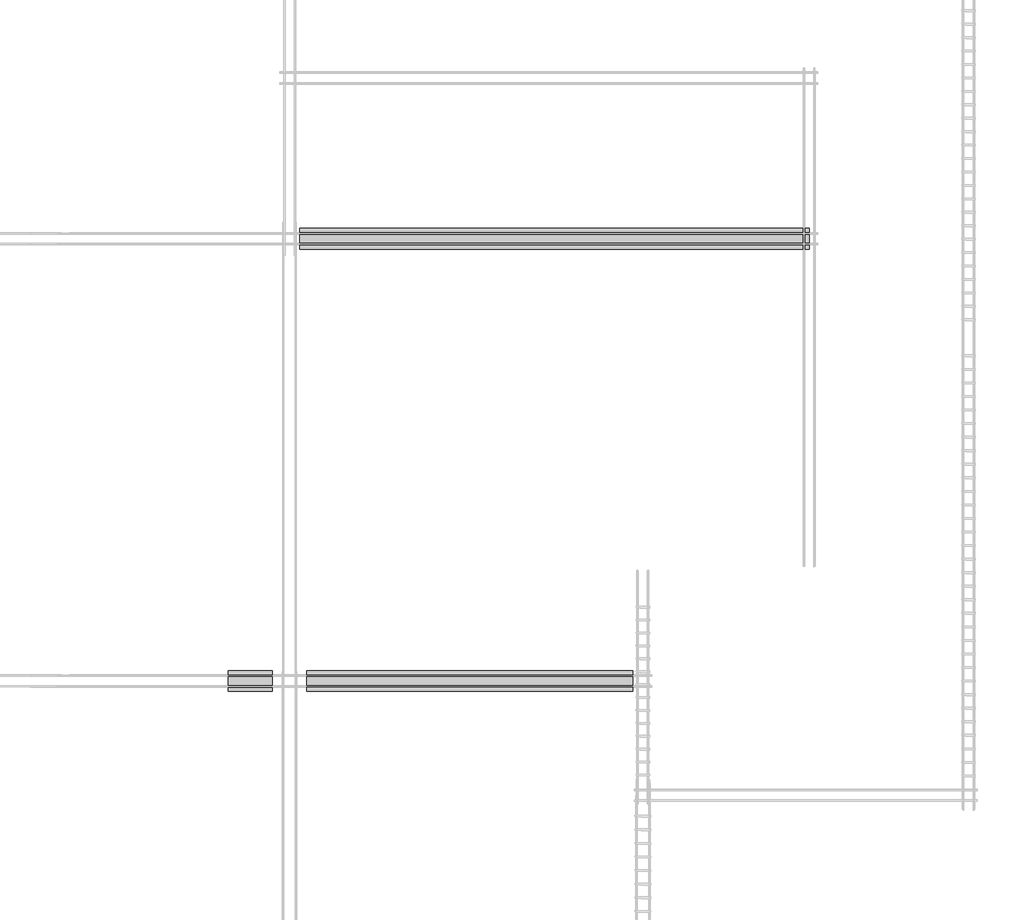
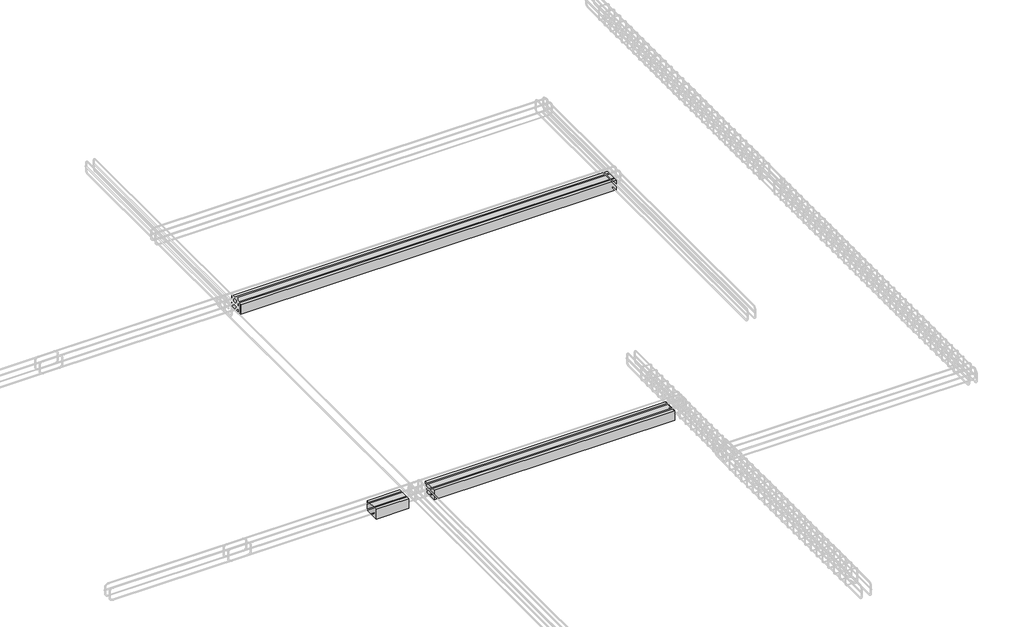
# One storey, part 1 of 5: 2 beams.
"""IFC4 building model written with IfcOpenShell, lengths in millimetres."""

from ifc_helpers import new_model, si_unit, frame, origin, place, context, project, spatial, polyline, outline, extrude, faceted_brep, element, save

model = new_model("IFC4")

# Units and contexts
model_context = context("Model", 3, world=origin())
ifc_project = project(units=[si_unit("LENGTHUNIT", "METRE", prefix="MILLI")], contexts=[model_context])

# Site, building, storey
site = spatial("IfcSite", under=ifc_project)
building = spatial("IfcBuilding", under=site)
storey = spatial("IfcBuildingStorey", under=building, Elevation=0.0)

# Beams
placement = place(None, origin())
element("IfcBeam", 1, ObjectType="Concrete-Rectangular Beam : 12 x 24", at=placement, inside=storey, context=model_context, shape_type="SweptSolid", body=[
    extrude(outline(polyline([(-6425.8418223, 5042.4251382), (-6425.8418223, 4813.8251382), (-10007.2418223, 4813.8251382), (-10007.2418223, 5042.4251382), (-6425.8418223, 5042.4251382)])), frame((0.0, 0.0, 152.4), z_axis=(0.0, 0.0, 1.0), x_axis=(1.0, 0.0, 0.0)), (0.0, 0.0, 1.0), 152.4),
    extrude(outline(polyline([(-10870.8418223, 4813.8251382), (-10870.8418223, 5042.4251382), (-10388.2418223, 5042.4251382), (-10388.2418223, 4813.8251382), (-10870.8418223, 4813.8251382)])), frame((0.0, 0.0, 152.4), z_axis=(0.0, 0.0, 1.0), x_axis=(1.0, 0.0, 0.0)), (0.0, 0.0, 1.0), 152.4),
])
element("IfcBeam", 2, ObjectType="Concrete-Rectangular Beam : 12 x 24", at=placement, inside=storey, context=model_context, shape_type="Brep", body=[
    faceted_brep([(-4482.7418223, 9678.3578802, 152.4), (-4482.7418223, 9906.9578802, 152.4), (-4482.7418223, 9906.9578802, 304.8), (-4482.7418223, 9678.3578802, 304.8), (-10083.4418223, 9678.3578802, 152.4), (-4597.0418223, 9678.3578802, 152.4), (-4597.0418223, 9678.3578802, 304.8), (-10083.4418223, 9678.3578802, 304.8), (-10083.4418223, 9906.9578802, 152.4), (-4597.0418223, 9906.9578802, 152.4), (-10083.4418223, 9906.9578802, 304.8), (-4597.0418223, 9906.9578802, 304.8)], [[[0, 1, 2, 3]], [[4, 5, 0, 3, 6, 7]], [[1, 0, 5, 4, 8, 9]], [[1, 9, 8, 10, 11, 2]], [[8, 4, 7, 10]], [[3, 2, 11, 10, 7, 6]]]),
])

save(model, "model.ifc")

# Revit data of these elements
# Type "Concrete-Rectangular Beam : 12 x 24"
#   Assembly Code = "B10"
#   Length [instance default] = 5' - 0"
#   b = 0' - 9"
#   h = 1' - 0"
#   Structural Material [instance default] = Concrete, Cast-in-Place gray
# Elements 1, 2 (IfcBeam, "Concrete-Rectangular Beam : 12 x 24")
#   Structural Material = Concrete, Cast-in-Place gray
#   Phase Created = New Construction
#   Materials on its faces: "Concrete, Cast-in-Place gray"
# Materials
#   "Concrete, Cast-in-Place gray": class "Concrete", colour RGB 192 192 192, transparency 0, Description = "Cast-in-place concrete", Cost = 0
